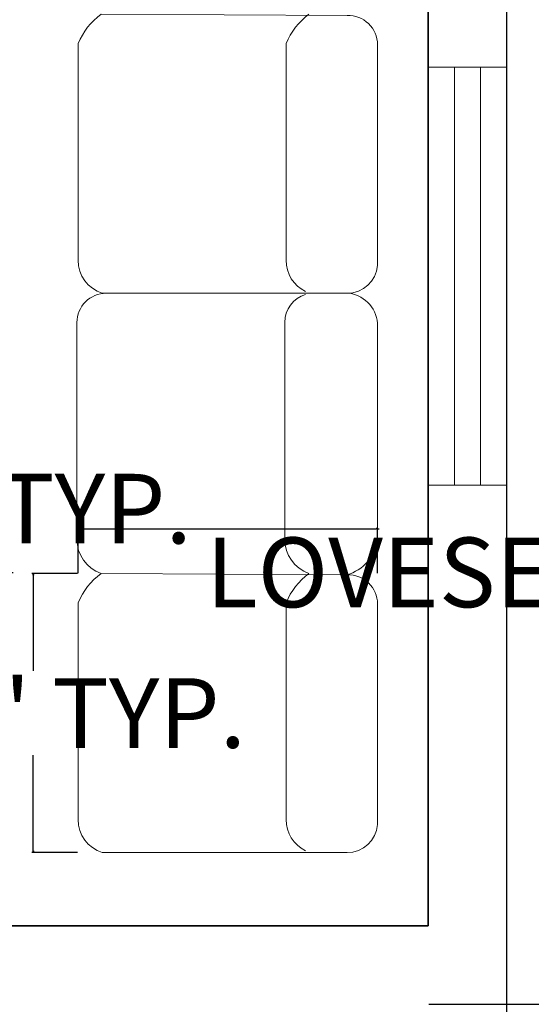
# Model space of a CAD drawing. Units: inches. Extents: x -11 to 443, y 65 to 743.
# Tile 4 of 10: x 276 to 335, y 212 to 325. Entities that reach past the tile are written whole.
import ezdxf

# ---------------------------------------------------------------- set-up
doc = ezdxf.new("R2010")
doc.units = ezdxf.units.IN
doc.header["$MEASUREMENT"] = 0
for name, color, linetype, lineweight in [('A-ANNO-DIMS', 2, 'Continuous', 18), ('A-GLAZ', 4, 'Continuous', 18), ('A-WALL', 7, 'Continuous', 35), ('C-PROP', 3, 'Continuous', 30), ('Furniture', 7, 'Continuous', 15)]:
    doc.layers.add(name, color=color, linetype=linetype, lineweight=lineweight)
doc.styles.get("Standard").update_dxf_attribs({"font": 'italic8.shx'})
doc.dimstyles.get("Standard").update_dxf_attribs({"dimtxt": 8, "dimasz": 0.18, "dimexe": 0.18, "dimexo": 0.0625, "dimgap": 0.09, "dimtad": 0, "dimtih": 1, "dimtoh": 1, "dimzin": 0, "dimdsep": 46, "dimlunit": 3, "dimtxsty": 'Standard', "dimblk": 'CLOSEDBLANK', "dimcen": 0.09, "dimclrd": 6, "dimclre": 5, "dimclrt": 4, "dimadec": 0, "dimazin": 0, "dimtfac": 1, "dimtofl": 0, "dimtmove": 0, "dimatfit": 3, "dimfxl": 1, "dimtolj": 1, "dimtzin": 0, "dimarcsym": 0})

# ---------------------------------------------------------------- blocks, each defined once
blk = doc.blocks.new('_ClosedBlank')
at = {"color": 0, "linetype": 'ByBlock', "lineweight": -2}
for p, q in [((-1, 0.167), (0, 0)), ((-1, 0.167), (-1, -0.167)), ((0, 0), (-1, -0.167))]:
    blk.add_line(p, q, dxfattribs=at)
blk = doc.blocks.new('*D6')
at = {"layer": 'A-ANNO-DIMS', "color": 0, "lineweight": -2, "transparency": 16777216}
for p, q in [((332.27, 706.92), (352.4, 706.92)), ((352.22, 706.74), (352.22, 411.77)), ((352.22, 107.1), (352.22, 402.07)), ((332.27, 106.92), (352.4, 106.92))]:
    blk.add_line(p, q, dxfattribs=at)
at = {"layer": 'Defpoints', "color": 0, "lineweight": 100, "transparency": 16777216}
for p in [(332.21, 706.92), (332.21, 106.92), (352.22, 106.92)]:
    blk.add_point(p, dxfattribs=at)
at = {"layer": 'A-ANNO-DIMS', "color": 0, "lineweight": -2, "transparency": 16777216, "xscale": 0.18, "yscale": 0.18, "zscale": 0.18}
for p, rotation in [((352.22, 706.92), 90), ((352.22, 106.92), 270)]:
    blk.add_blockref('_ClosedBlank', p, dxfattribs=dict(at, rotation=rotation))
at = {"layer": 'A-ANNO-DIMS', "color": 0, "transparency": 16777216, "insert": (352.22, 406.92), "char_height": 8, "attachment_point": 5}
blk.add_mtext("\\A1;50'", dxfattribs=at)
blk = doc.blocks.new('WIN-48x9')
for p, q in [((0, 48), (0, 0)), ((9, 48), (0, 48)), ((3, 0), (3, 48)), ((6, 0), (6, 48)), ((9, 0), (9, 48)), ((0, 0), (9, 0))]:
    blk.add_line(p, q)
blk = doc.blocks.new('SECTIONAL-SEAT')
for p, q in [((30.86, 31.9, -13.5), (2.62, 32.04, -13.5)), ((0, 28.69, -13.5), (0, 3.79, -13.5)), ((23.85, 28.69, -13.5), (23.85, 3.79, -13.5)), ((34.36, 3.2, -13.5), (34.36, 28.55, -13.5)), ((2.77, 0, -13.5), (30.86, 0, -13.5))]:
    blk.add_line(p, q)
for centre, radius, start, end in [((7.52, 25.51, -13.5), 8.17, 126.8838, 157.0502), ((31.38, 25.51, -13.5), 8.17, 126.8838, 157.0502), ((31, 28.55, -13.5), 3.35, 0, 92.4088), ((3.97, 3.79, -13.5), 3.98, 180, 252.2888), ((27.83, 3.79, -13.5), 3.98, 180, 244.0743), ((30.86, 3.51, -13.5), 3.51, 270, 355.0498)]:
    blk.add_arc(centre, radius, start, end)
blk = doc.blocks.new('*D22')
at = {"layer": 'A-ANNO-DIMS', "color": 5, "lineweight": -2, "transparency": 16777216}
for p, q in [((161.71, 263.5), (161.71, 269.02)), ((197.71, 263.5), (197.71, 269.02))]:
    blk.add_line(p, q, dxfattribs=at)
at = {"layer": 'A-ANNO-DIMS', "color": 6, "lineweight": -2, "transparency": 16777216}
for p, q in [((161.89, 268.84), (197.53, 268.84)), ((197.71, 268.84), (197.89, 268.84))]:
    blk.add_line(p, q, dxfattribs=at)
at = {"layer": 'Defpoints', "color": 0, "lineweight": 100, "transparency": 16777216}
for p in [(197.71, 268.84), (161.71, 263.44), (197.71, 263.44)]:
    blk.add_point(p, dxfattribs=at)
at = {"layer": 'A-ANNO-DIMS', "color": 6, "lineweight": -2, "transparency": 16777216, "xscale": 0.18, "yscale": 0.18, "zscale": 0.18, "rotation": 180}
blk.add_blockref('_ClosedBlank', (161.71, 268.84), dxfattribs=at)
at = {"layer": 'A-ANNO-DIMS', "color": 6, "lineweight": -2, "transparency": 16777216, "xscale": 0.18, "yscale": 0.18, "zscale": 0.18}
blk.add_blockref('_ClosedBlank', (197.71, 268.84), dxfattribs=at)
at = {"layer": 'A-ANNO-DIMS', "color": 4, "transparency": 16777216, "insert": (255.12, 268.84), "char_height": 8, "attachment_point": 5}
blk.add_mtext('\\A1;DOOR 3\'-0" TYP.', dxfattribs=at)
blk = doc.blocks.new('*D32')
at = {"layer": 'A-ANNO-DIMS', "color": 5, "lineweight": -2, "transparency": 16777216}
for p, q in [((223.42, 253.79), (223.42, 261.7)), ((275.39, 253.79), (275.39, 261.7))]:
    blk.add_line(p, q, dxfattribs=at)
at = {"layer": 'A-ANNO-DIMS', "color": 6, "lineweight": -2, "transparency": 16777216}
for p, q in [((223.6, 261.52), (275.21, 261.52)), ((275.39, 261.52), (275.57, 261.52))]:
    blk.add_line(p, q, dxfattribs=at)
at = {"layer": 'Defpoints', "color": 0, "lineweight": 100, "transparency": 16777216}
for p in [(275.39, 261.52), (223.42, 253.72), (275.39, 253.72)]:
    blk.add_point(p, dxfattribs=at)
at = {"layer": 'A-ANNO-DIMS', "color": 6, "lineweight": -2, "transparency": 16777216, "xscale": 0.18, "yscale": 0.18, "zscale": 0.18, "rotation": 180}
blk.add_blockref('_ClosedBlank', (223.42, 261.52), dxfattribs=at)
at = {"layer": 'A-ANNO-DIMS', "color": 6, "lineweight": -2, "transparency": 16777216, "xscale": 0.18, "yscale": 0.18, "zscale": 0.18}
blk.add_blockref('_ClosedBlank', (275.39, 261.52), dxfattribs=at)
at = {"layer": 'A-ANNO-DIMS', "color": 4, "transparency": 16777216, "insert": (349.75, 261.52), "char_height": 8, "attachment_point": 5}
blk.add_mtext('\\A1;LOVESEAT 4\'-4" TYP.', dxfattribs=at)
blk = doc.blocks.new('*D34')
at = {"layer": 'A-ANNO-DIMS', "color": 5, "lineweight": -2, "transparency": 16777216}
for p, q in [((283.03, 261.45), (283.03, 266.72)), ((317.39, 261.45), (317.39, 266.72))]:
    blk.add_line(p, q, dxfattribs=at)
at = {"layer": 'A-ANNO-DIMS', "color": 6, "lineweight": -2, "transparency": 16777216}
for p, q in [((283.21, 266.54), (317.21, 266.54)), ((317.39, 266.54), (317.57, 266.54))]:
    blk.add_line(p, q, dxfattribs=at)
at = {"layer": 'Defpoints', "color": 0, "lineweight": 100, "transparency": 16777216}
for p in [(317.39, 266.54), (283.03, 261.39), (317.39, 261.39)]:
    blk.add_point(p, dxfattribs=at)
at = {"layer": 'A-ANNO-DIMS', "color": 6, "lineweight": -2, "transparency": 16777216, "xscale": 0.18, "yscale": 0.18, "zscale": 0.18, "rotation": 180}
blk.add_blockref('_ClosedBlank', (283.03, 266.54), dxfattribs=at)
at = {"layer": 'A-ANNO-DIMS', "color": 6, "lineweight": -2, "transparency": 16777216, "xscale": 0.18, "yscale": 0.18, "zscale": 0.18}
blk.add_blockref('_ClosedBlank', (317.39, 266.54), dxfattribs=at)
at = {"layer": 'A-ANNO-DIMS', "color": 4, "transparency": 16777216, "insert": (392.9, 266.54), "char_height": 8, "attachment_point": 5}
blk.add_mtext('\\A1;SEAT 2\'-10 1/2" TYP.', dxfattribs=at)
blk = doc.blocks.new('*D35')
at = {"layer": 'A-ANNO-DIMS', "color": 5, "lineweight": -2, "transparency": 16777216}
for p, q in [((282.97, 261.39), (277.7, 261.39)), ((282.97, 229.35), (277.7, 229.35))]:
    blk.add_line(p, q, dxfattribs=at)
at = {"layer": 'A-ANNO-DIMS', "color": 6, "lineweight": -2, "transparency": 16777216}
for p, q in [((277.88, 261.21), (277.88, 250.22)), ((277.88, 229.53), (277.88, 240.52))]:
    blk.add_line(p, q, dxfattribs=at)
at = {"layer": 'Defpoints', "color": 0, "lineweight": 100, "transparency": 16777216}
for p in [(277.88, 261.39), (283.03, 261.39), (283.03, 229.35)]:
    blk.add_point(p, dxfattribs=at)
at = {"layer": 'A-ANNO-DIMS', "color": 6, "lineweight": -2, "transparency": 16777216, "xscale": 0.18, "yscale": 0.18, "zscale": 0.18}
for p, rotation in [((277.88, 261.39), 90), ((277.88, 229.35), 270)]:
    blk.add_blockref('_ClosedBlank', p, dxfattribs=dict(at, rotation=rotation))
at = {"layer": 'A-ANNO-DIMS', "color": 4, "transparency": 16777216, "insert": (277.88, 245.37), "char_height": 8, "attachment_point": 5}
blk.add_mtext('\\A1;2\'-8" TYP.', dxfattribs=at)
blk = doc.blocks.new('*D36')
at = {"layer": 'A-ANNO-DIMS', "color": 5, "lineweight": -2, "transparency": 16777216}
for p, q in [((323.27, 625.92), (362.85, 625.92)), ((323.27, 211.92), (362.85, 211.92))]:
    blk.add_line(p, q, dxfattribs=at)
at = {"layer": 'A-ANNO-DIMS', "color": 6, "lineweight": -2, "transparency": 16777216}
for p, q in [((362.67, 625.74), (362.67, 423.77)), ((362.67, 212.1), (362.67, 414.07))]:
    blk.add_line(p, q, dxfattribs=at)
at = {"layer": 'Defpoints', "color": 0, "lineweight": 100, "transparency": 16777216}
for p in [(323.21, 625.92), (362.67, 625.92), (323.21, 211.92)]:
    blk.add_point(p, dxfattribs=at)
at = {"layer": 'A-ANNO-DIMS', "color": 6, "lineweight": -2, "transparency": 16777216, "xscale": 0.18, "yscale": 0.18, "zscale": 0.18}
for p, rotation in [((362.67, 625.92), 90), ((362.67, 211.92), 270)]:
    blk.add_blockref('_ClosedBlank', p, dxfattribs=dict(at, rotation=rotation))
at = {"layer": 'A-ANNO-DIMS', "color": 4, "transparency": 16777216, "insert": (362.67, 418.92), "char_height": 8, "attachment_point": 5}
blk.add_mtext('\\A1;34\'-6"', dxfattribs=at)

msp = doc.modelspace()

# ---------------------------------------------------------------- linework, layer by layer
at = {"layer": 'A-WALL'}
for p, q in [((323.209, 220.92), (323.209, 373.92)), ((166.209, 220.92), (323.209, 220.92))]:
    msp.add_line(p, q, dxfattribs=at)
at = {"layer": 'C-PROP'}
msp.add_lwpolyline([(44.209, 106.92), (332.209, 106.92), (332.209, 706.92), (44.209, 706.92)], close=True, dxfattribs=at)
at = {"layer": 'Furniture'}
for p, q in [((314.187, 293.579, -13.498), (286.235, 293.579, -13.498)), ((282.887, 290.229, -13.498), (282.887, 271.586, -13.498)), ((306.738, 290.229, -13.498), (306.738, 271.586, -13.498)), ((317.389, 265.177, -13.498), (317.389, 289.792, -13.498)), ((282.887, 271.586, -13.498), (282.887, 265.323, -13.498)), ((306.738, 271.586, -13.498), (306.738, 265.323, -13.498))]:
    msp.add_line(p, q, dxfattribs=at)
for centre, radius, start, end in [((286.235, 290.231, -13.498), 3.348, 90, 180.02896), ((310.086, 290.231, -13.498), 3.348, 106.75774, 180.02896), ((313.549, 289.792, -13.498), 3.84, 0, 80.44416), ((287.066, 265.323, -13.498), 4.179, 180, 250.24112), ((310.916, 265.323, -13.498), 4.179, 180, 250.24112), ((312.509, 265.994, -13.498), 4.948, 286.26799, 350.49369)]:
    msp.add_arc(centre, radius, start, end, dxfattribs=at)

# ---------------------------------------------------------------- block references
at = {"layer": 'A-GLAZ'}
msp.add_blockref('WIN-48x9', (323.209, 271.525), dxfattribs=at)
at = {"layer": 'Furniture'}
for p in [(283.033, 293.573), (283.033, 229.346)]:
    msp.add_blockref('SECTIONAL-SEAT', p, dxfattribs=at)

# ---------------------------------------------------------------- dimensions: what is measured, and where the dimension line sits
at = {"layer": 'A-ANNO-DIMS'}
for base, p1, p2, override, picture, middle in [((352.221, 106.92), (332.209, 706.92), (332.209, 106.92), {"dimclrd": 0, "dimclre": 0, "dimclrt": 0}, '*D6', (352.221, 406.92)), ((362.669, 625.92), (323.209, 211.92), (323.209, 625.92), {"dimdec": 1, "dimlfac": 1, "dimrnd": 0, "dimzin": 1, "dimdsep": 46, "dimlunit": 4, "dimfrac": 2}, '*D36', (362.669, 418.92))]:
    dim = msp.add_linear_dim(base=base, p1=p1, p2=p2, angle=90, dimstyle='Standard', override=override, dxfattribs=at)
    dim.commit()
    dim.dimension.update_dxf_attribs({"geometry": picture, "text_midpoint": middle})
for base, p1, p2, text, picture, middle in [((317.389, 266.543), (283.033, 261.39), (317.389, 261.39), 'SEAT <> TYP.', '*D34', (392.897, 266.543)), ((197.709, 268.842), (161.709, 263.442), (197.709, 263.442), 'DOOR <> TYP.', '*D22', (255.122, 268.842)), ((275.388, 261.518), (223.42, 253.723), (275.388, 253.723), 'LOVESEAT <> TYP.', '*D32', (349.753, 261.518))]:
    dim = msp.add_linear_dim(base=base, p1=p1, p2=p2, text=text, dimstyle='Standard', override={"dimdec": 1, "dimlfac": 1, "dimrnd": 0, "dimzin": 1, "dimdsep": 46, "dimlunit": 4, "dimfrac": 2}, dxfattribs=at)
    dim.commit()
    dim.dimension.update_dxf_attribs({"geometry": picture, "text_midpoint": middle})
dim = msp.add_linear_dim(base=(277.879, 261.39), p1=(283.033, 229.346), p2=(283.033, 261.39), angle=90, text='<> TYP.', dimstyle='Standard', override={"dimdec": 1, "dimlfac": 1, "dimrnd": 0, "dimzin": 1, "dimdsep": 46, "dimlunit": 4, "dimfrac": 2}, dxfattribs=at)
dim.commit()
dim.dimension.update_dxf_attribs({"geometry": '*D35', "text_midpoint": (277.879, 245.368)})

doc.saveas('drawing.dxf')
